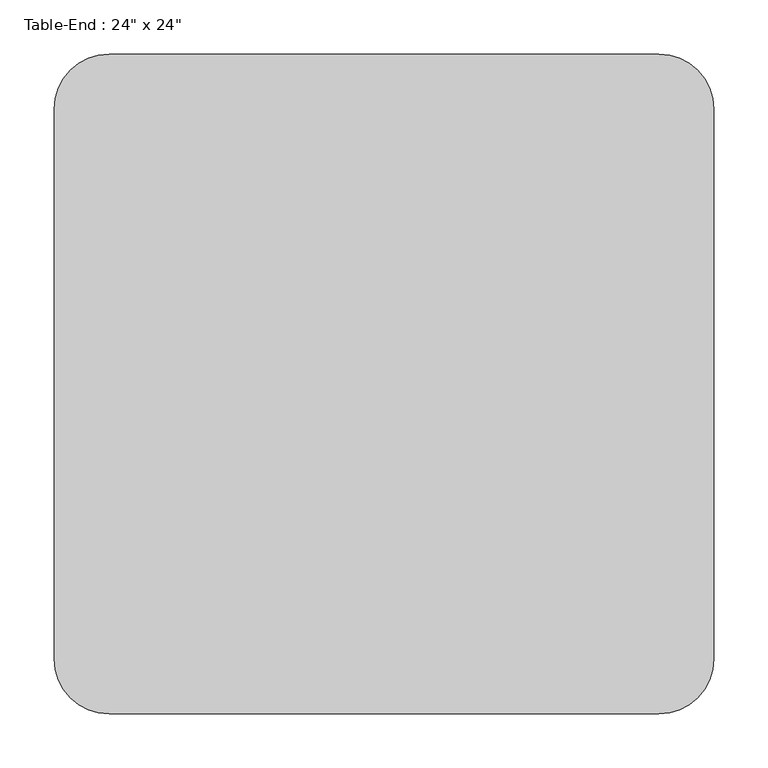
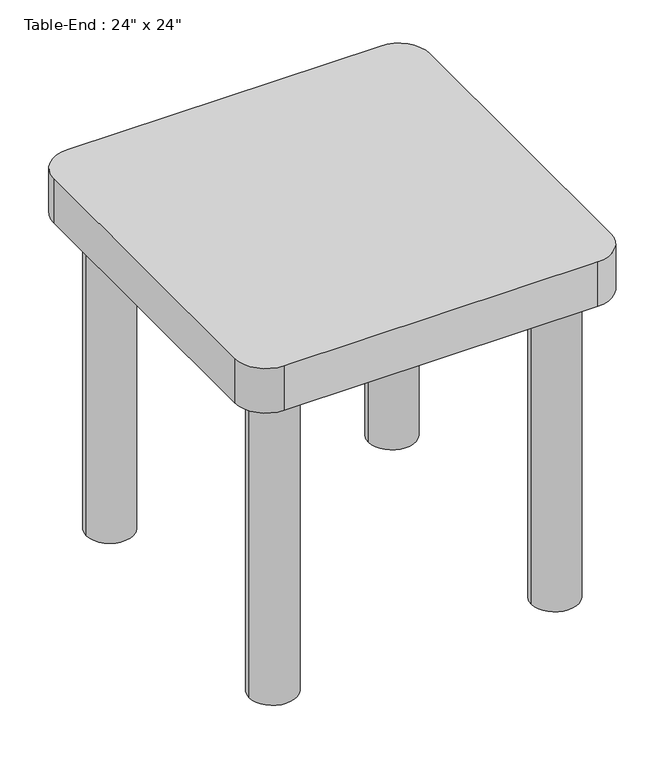
"""IFC4 building model written with IfcOpenShell, lengths in millimetres: furniture geometry."""

from ifc_helpers import new_model, si_unit, point, frame, frame_2d, origin, origin_with_axes, place, context, project, spatial, polyline, circle_curve, trimmed, segment, composite_curve, outline, extrude, source, transform, mapped, element, save


def furniture_31d08a24(model_context):
    return source(origin(), model_context, "Body", "SweptSolid", [
        extrude(outline(composite_curve([segment(polyline([(562.5336303, -152.4), (54.5336303, -152.4)]), True, "CONTINUOUS"), segment(trimmed(circle_curve(frame_2d((54.5336303, -101.6)), 50.8), [point((54.5336303, -152.4))], [point((3.7336303, -101.6))], False, "CARTESIAN"), True, "CONTINUOUS"), segment(polyline([(3.7336303, -101.6), (3.7336303, 406.4)]), True, "CONTINUOUS"), segment(trimmed(circle_curve(frame_2d((54.5336303, 406.4)), 50.8), [point((3.7336303, 406.4))], [point((54.5336303, 457.2))], False, "CARTESIAN"), True, "CONTINUOUS"), segment(polyline([(54.5336303, 457.2), (562.5336303, 457.2)]), True, "CONTINUOUS"), segment(trimmed(circle_curve(frame_2d((562.5336303, 406.4)), 50.8), [point((562.5336303, 457.2))], [point((613.3336303, 406.4))], False, "CARTESIAN"), True, "CONTINUOUS"), segment(polyline([(613.3336303, 406.4), (613.3336303, -101.6)]), True, "CONTINUOUS"), segment(trimmed(circle_curve(frame_2d((562.5336303, -101.6)), 50.8), [point((613.3336303, -101.6))], [point((562.5336303, -152.4))], False, "CARTESIAN"), True, "CONTINUOUS")], self_intersect=False)), frame((0.0, 0.0, 533.4), z_axis=(0.0, 0.0, 1.0), x_axis=(1.0, 0.0, 0.0)), (0.0, 0.0, 1.0), 76.2),
        extrude(outline(composite_curve([segment(trimmed(circle_curve(frame_2d((79.9336303, 381.0)), 38.1), [point((41.8336303, 381.0))], [point((118.0336303, 381.0))], False, "CARTESIAN"), True, "CONTINUOUS"), segment(trimmed(circle_curve(frame_2d((79.9336303, 381.0)), 38.1), [point((118.0336303, 381.0))], [point((41.8336303, 381.0))], False, "CARTESIAN"), True, "CONTINUOUS")], self_intersect=False)), origin_with_axes(), (0.0, 0.0, 1.0), 533.4),
        extrude(outline(composite_curve([segment(trimmed(circle_curve(frame_2d((79.9336303, -76.2)), 38.1), [point((41.8336303, -76.2))], [point((118.0336303, -76.2))], False, "CARTESIAN"), True, "CONTINUOUS"), segment(trimmed(circle_curve(frame_2d((79.9336303, -76.2)), 38.1), [point((118.0336303, -76.2))], [point((41.8336303, -76.2))], False, "CARTESIAN"), True, "CONTINUOUS")], self_intersect=False)), origin_with_axes(), (0.0, 0.0, 1.0), 533.4),
        extrude(outline(composite_curve([segment(trimmed(circle_curve(frame_2d((537.1336303, -76.2)), 38.1), [point((499.0336303, -76.2))], [point((575.2336303, -76.2))], False, "CARTESIAN"), True, "CONTINUOUS"), segment(trimmed(circle_curve(frame_2d((537.1336303, -76.2)), 38.1), [point((575.2336303, -76.2))], [point((499.0336303, -76.2))], False, "CARTESIAN"), True, "CONTINUOUS")], self_intersect=False)), origin_with_axes(), (0.0, 0.0, 1.0), 533.4),
        extrude(outline(composite_curve([segment(trimmed(circle_curve(frame_2d((537.1336303, 381.0)), 38.1), [point((499.0336303, 381.0))], [point((575.2336303, 381.0))], False, "CARTESIAN"), True, "CONTINUOUS"), segment(trimmed(circle_curve(frame_2d((537.1336303, 381.0)), 38.1), [point((575.2336303, 381.0))], [point((499.0336303, 381.0))], False, "CARTESIAN"), True, "CONTINUOUS")], self_intersect=False)), origin_with_axes(), (0.0, 0.0, 1.0), 533.4),
    ])


if __name__ == "__main__":
    model = new_model("IFC4")
    model_context = context("Model", 3, world=origin())
    ifc_project = project(units=[si_unit("LENGTHUNIT", "METRE", prefix="MILLI")], contexts=[model_context])
    site = spatial("IfcSite", under=ifc_project)
    building = spatial("IfcBuilding", under=site)
    placement = place(None, origin())
    furniture_shape = furniture_31d08a24(model_context)
    element("IfcFurniture", 1, ObjectType="Table-End : 24\" x 24\"", at=placement, inside=building, context=model_context, shape_type="MappedRepresentation", body=[
        mapped(furniture_shape, transform((0.0, 0.0, 0.0), x_axis=(1.0, 0.0, 0.0), y_axis=(0.0, 1.0, 0.0), z_axis=(0.0, 0.0, 1.0))),
    ])
    save(model, "model.ifc")

# Revit data of these elements
# Type "Table-End : 24\" x 24\""
#   Assembly Code = "E2020200"
#   Height = 2' - 0"
#   Length = 2' - 0"
#   Width = 2' - 0"
#   Base Material = Birch
#   Top Material = Laminate, Ivory, Matte
#   Default Elevation = 0
# Element 1 (IfcFurniture, "Table-End : 24\" x 24\"")
#   Materials on its faces: "Laminate, Ivory, Matte", "Birch"
# Materials
#   "Birch": class "Wood", colour RGB 210 159 95, transparency 0, Description = "Betula Alleghaniensis", Cost = 0
#   "Laminate, Ivory, Matte": class "Plastic", colour RGB 247 247 239, transparency 0, Description = "Plastic Laminate - Ivory, Matte", Cost = 0
